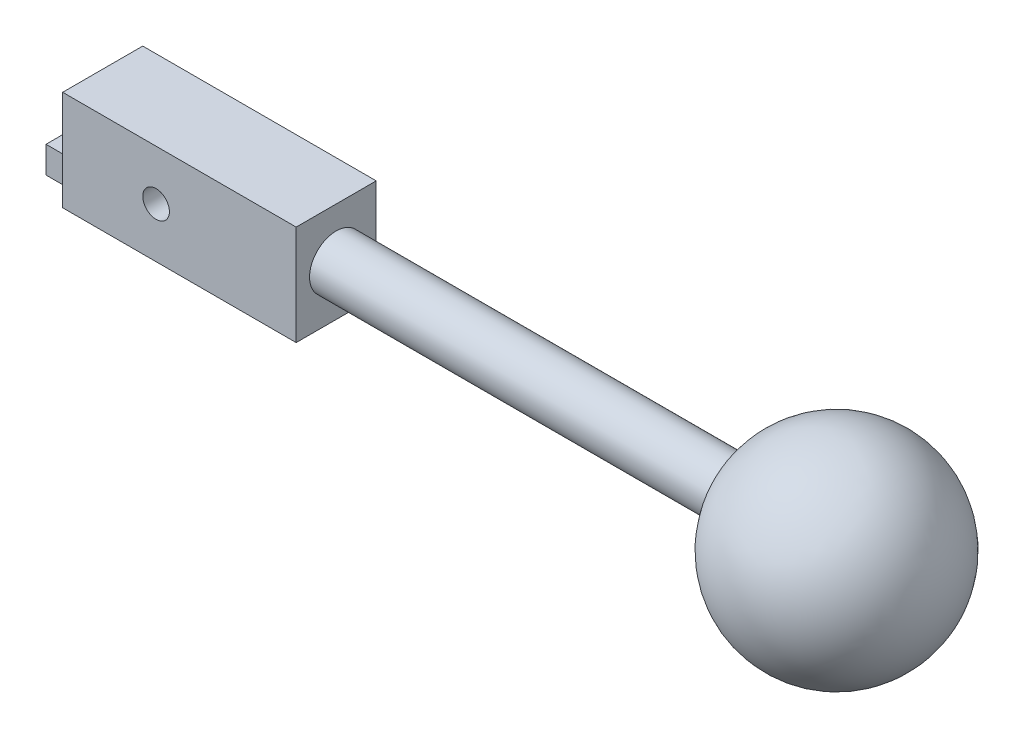
SolidWorks part; units mm, degrees
material "Plain Carbon Steel"
ref_plane "Front Plane" through (0, 0, 0) normal (0, 0, 1) x (1, 0, 0)
ref_plane "Top Plane" through (0, 0, 0) normal (0, 1, 0) x (1, 0, 0)
ref_plane "Right Plane" through (0, 0, 0) normal (1, 0, 0) x (0, 0, -1)
sketch "Hub Block Sketch" plane through (0, 0, 0) normal (0, 0, 1) x (1, 0, 0)
  line L1 (-17.5, -7.5) -> (17.5, -7.5)
  line L2 (-17.5, -7.5) -> (-17.5, 7.5)
  line L3 (-17.5, 7.5) -> (17.5, 7.5)
  line L4 (17.5, -7.5) -> (17.5, 7.5)
  line L5 (-17.5, -7.5) -> (17.5, 7.5) construction
  line L6 (-17.5, 7.5) -> (17.5, -7.5) construction
  point P0 (0, 0)
  dimension "D1" = 15
  dimension "D2" = 35
extrude "Hub Block" add sketch "Hub Block Sketch" along normal blind 12
sketch "Drive Tab Sketch" plane through (-17.5, 0, 0) normal (-1, 0, 0) x (0, 0, 1)
  line L0 (12, -7.5) -> (0, -7.5) construction
  line L1 (3, -7.5) -> (9, -7.5)
  line L2 (3, -7.5) -> (3, -3.5)
  line L3 (3, -3.5) -> (9, -3.5)
  line L4 (9, -7.5) -> (9, -3.5)
  line L5 (12, 7.5) -> (0, 7.5) construction
  point P6 (6, -7.5)
  point P9 (6, 7.5)
  dimension "D1" = 6
  dimension "D2" = 4
extrude "Drive Tab" add sketch "Drive Tab Sketch" along normal blind 5.5
sketch "Shaft Sketch" plane through (17.5, 0, 0) normal (1, 0, 0) x (0, 0, -1)
  line L0 (-12, 7.5) -> (0, 7.5) construction
  circle A0 centre (-6, 0) radius 4
  point P5 (-6, 7.5)
  dimension "D1" = 8
extrude "Shaft Ø8" add sketch "Shaft Sketch" along normal blind 75
sketch "Ball Knob Sketch" plane through (0, 0, 0) normal (0, 1, 0) x (1, 0, 0)
  line L0 (92.5, 0) -> (92.5, -18.2173) construction
  line L2 (92.5, -10) -> (92.5, -2) construction
  line L3 (17.5, -12) -> (17.5, 0) construction
  line L4 (92.5, 9) -> (92.5, -21)
  arc A0 (92.5, 9) -> (92.5, -21) centre (92.5, -6) cw
  point P10 (17.5, -6)
  dimension "D2" = 15
  dimension "D1" = 30
revolve "Ball Knob Ø30" add sketch "Ball Knob Sketch" angle 360 about L0
sketch "Pin Hole Sketch" plane through (0, 0, 12) normal (0, 0, 1) x (1, 0, 0)
  line L0 (-17.5, 7.5) -> (-17.5, -7.5) construction
  circle A0 centre (-3.5, 0) radius 2
  point P5 (-17.5, 0)
  dimension "D1" = 4
  dimension "D2" = 14
extrude "Pin Hole Ø4" cut sketch "Pin Hole Sketch" against normal blind 75
